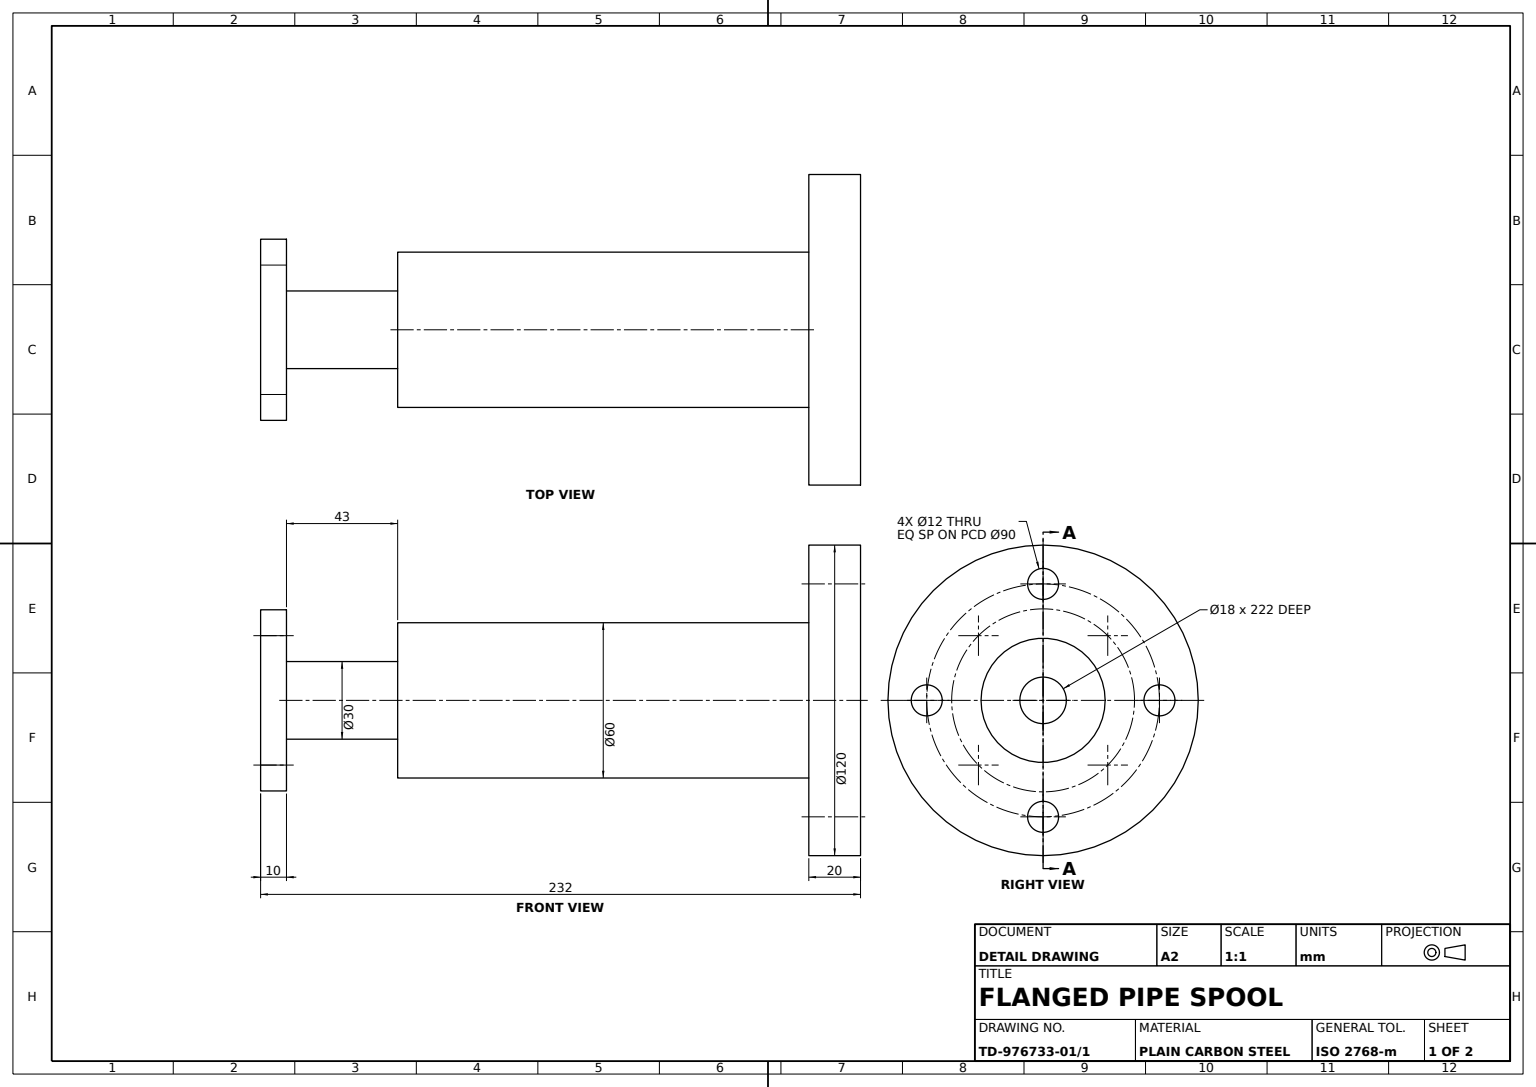
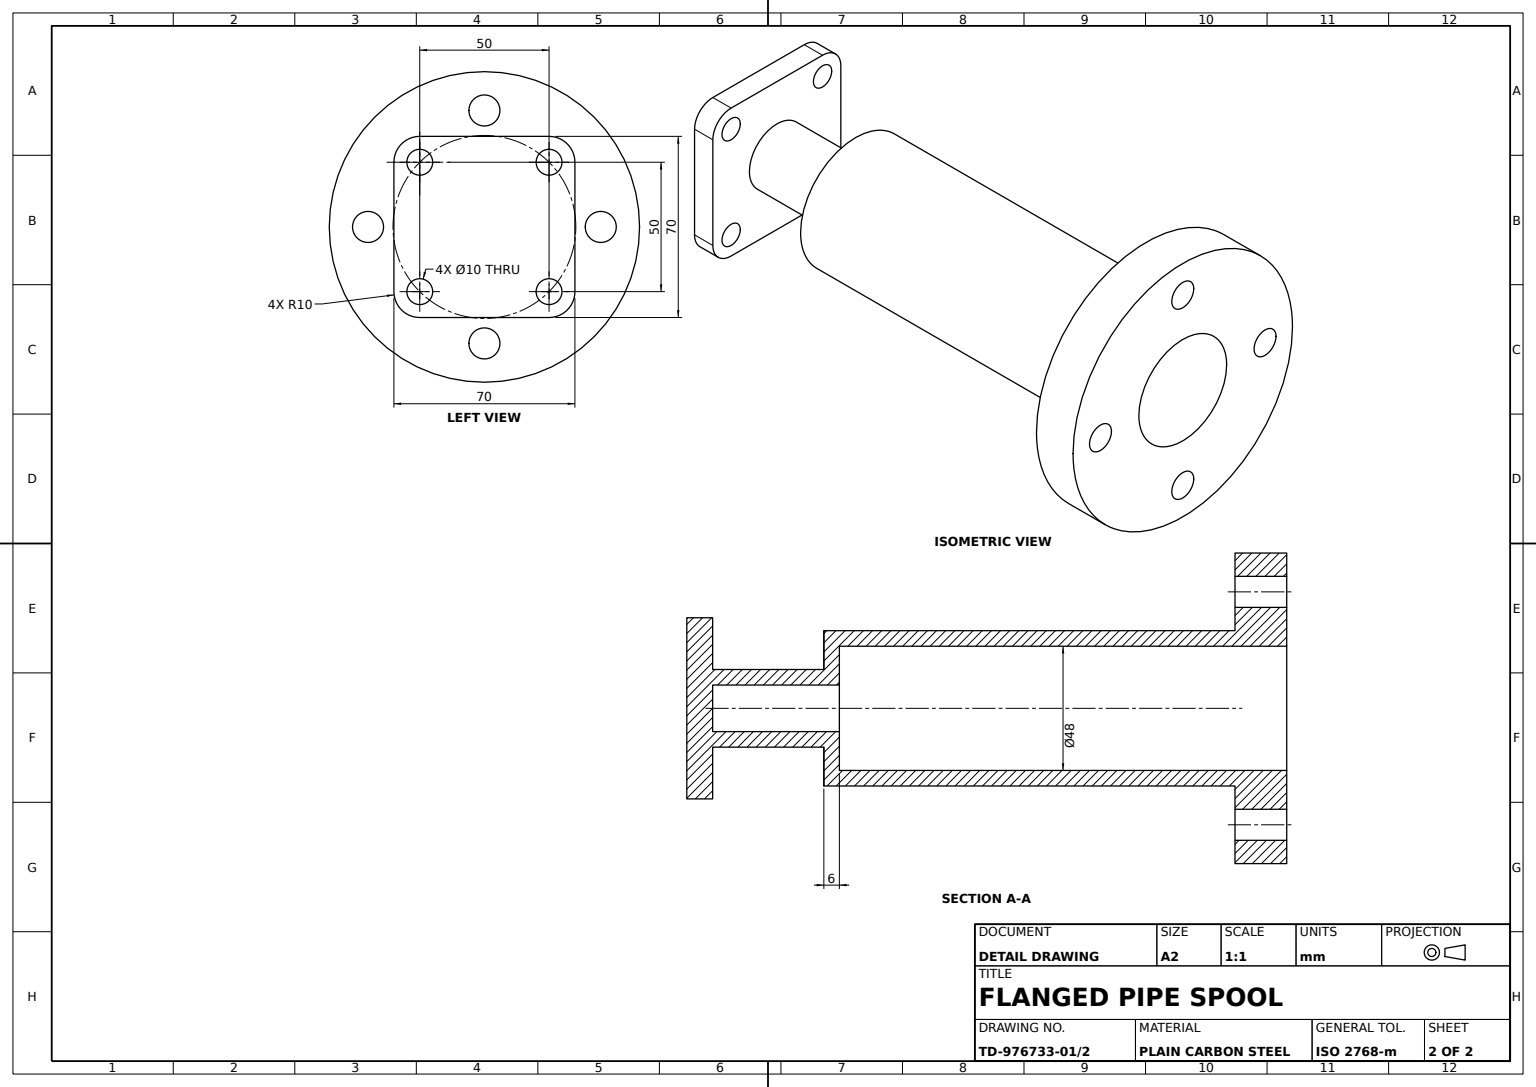
SolidWorks part; units mm, degrees
material "Plain Carbon Steel"
ref_plane "Front Plane" through (0, 0, 0) normal (0, 0, 1) x (1, 0, 0)
ref_plane "Top Plane" through (0, 0, 0) normal (0, 1, 0) x (1, 0, 0)
ref_plane "Right Plane" through (0, 0, 0) normal (1, 0, 0) x (0, 0, -1)
sketch "Housing Profile Sketch" plane through (0, 0, 0) normal (0, 0, 1) x (1, 0, 0)
  line L0 (0, 15) -> (43, 15)
  line L1 (43, 15) -> (43, 30)
  line L2 (43, 30) -> (202, 30)
  line L3 (202, 30) -> (202, 60)
  line L4 (202, 60) -> (222, 60)
  line L5 (222, 60) -> (222, 24)
  line L6 (222, 24) -> (49, 24)
  line L7 (49, 24) -> (49, 9)
  line L8 (49, 9) -> (0, 9)
  line L9 (0, 9) -> (0, 15)
  line L10 (0, 0) -> (118.6075, 0) construction
  dimension "D1" = 9
  dimension "D2" = 15
  dimension "D3" = 24
  dimension "D4" = 30
  dimension "D5" = 60
  dimension "D6" = 20
  dimension "D7" = 222
  dimension "D8" = 6
  dimension "D9" = 43
  dimension "D10" = 6
revolve "Housing Body Revolve" add sketch "Housing Profile Sketch" angle 360 about L10
sketch "Square Flange Sketch 70x70" plane through (0, 0, 0) normal (-1, 0, 0) x (0, 0, 1)
  line L1 (-35, 35) -> (35, 35)
  line L2 (-35, 35) -> (-35, -35)
  line L3 (-35, -35) -> (35, -35)
  line L4 (35, 35) -> (35, -35)
  line L5 (-35, 35) -> (35, -35) construction
  line L6 (-35, -35) -> (35, 35) construction
  point P0 (0, 0)
  dimension "D1" = 70
  dimension "D2" = 70
extrude "Square Mounting Flange" add sketch "Square Flange Sketch 70x70" along normal blind 10
fillet "Square Flange Corner Fillets R10" radius 10 4 edges at (-5, -35, -35) (-5, -35, 35) (-5, 35, 35) (-5, 35, -35)
sketch "Square Flange Holes Sketch" plane through (-10, 0, 0) normal (-1, 0, 0) x (0, 0, 1)
  circle A0 centre (25, 25) radius 5
  circle A1 centre (-25, 25) radius 5
  circle A2 centre (-25, -25) radius 5
  circle A3 centre (25, -25) radius 5
  dimension "D1" = 10
  dimension "D2" = 10
  dimension "D3" = 10
  dimension "D4" = 10
extrude "Square Flange Mounting Holes 4x" cut sketch "Square Flange Holes Sketch" against normal blind 10
sketch "Round Flange Hole Sketch" plane through (202, 0, 0) normal (-1, 0, 0) x (0, 0, 1)
  circle A0 centre (45, 0) radius 6
  circle A1 centre (0, 0) radius 30 construction
  dimension "D1" = 12
  dimension "D2" = 45
  dimension "D3" = 45
extrude "Round Flange Bolt Hole Ø12" cut sketch "Round Flange Hole Sketch" against normal through all
pattern_circular "Round Flange Bolt Hole Pattern 4x" count 4 over 360 about axis through (0, 0, 0) along (1, 0, 0) of "Round Flange Bolt Hole Ø12"
